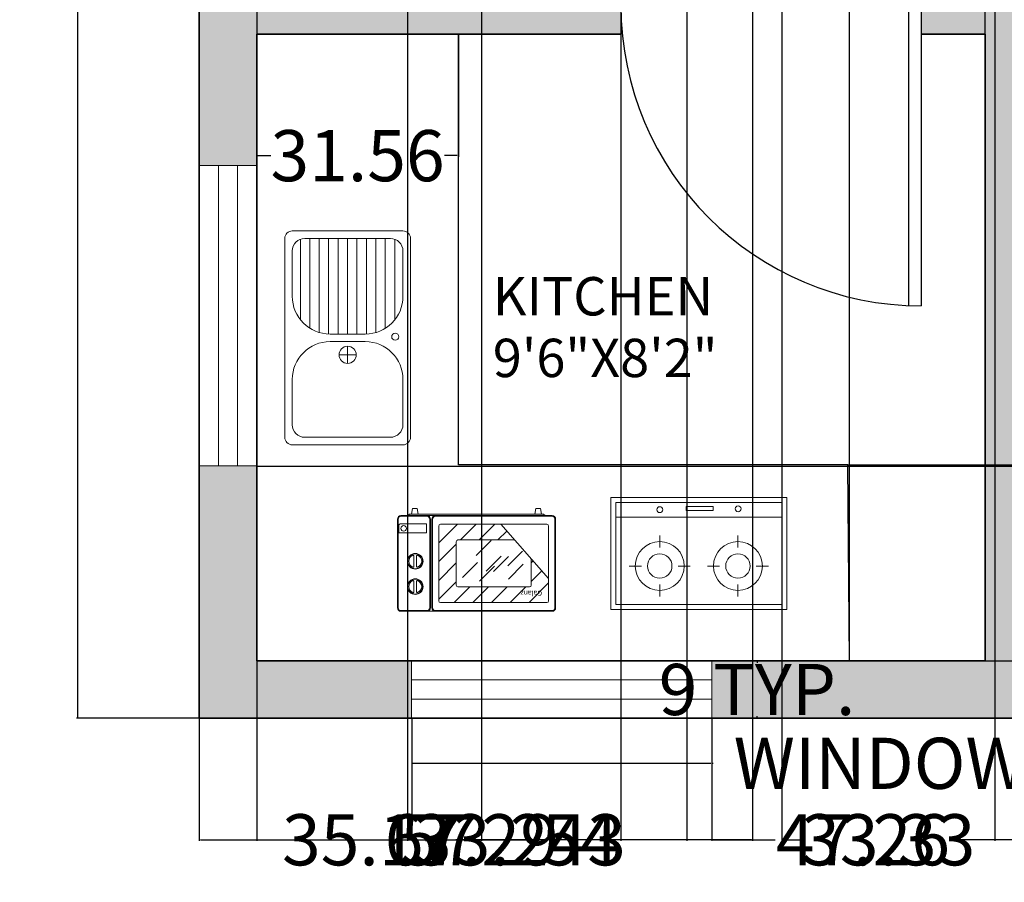
# Model space of a CAD drawing. Units: inches. Extents: x -24 to 368, y -370 to 58.
# Tile 1 of 9: x -24 to 130, y -370 to -235. Entities that reach past the tile are written whole.
import ezdxf

# ---------------------------------------------------------------- set-up
doc = ezdxf.new("R2010")
doc.units = ezdxf.units.IN
doc.header["$MEASUREMENT"] = 0
for name, color, linetype, lineweight in [('A-ANNO-DIMS', 2, 'Continuous', 18), ('A-AREA-IDEN', 7, 'Continuous', 18), ('A-EQPM', 7, 'Continuous', 15), ('A-EQPM-PATT', 7, 'Continuous', 15), ('A-FLOR-FIXT', 8, 'Continuous', 18), ('A-WALL', 7, 'Continuous', 35)]:
    doc.layers.add(name, color=color, linetype=linetype, lineweight=lineweight)
for name, color, linetype, lineweight, true_color in [('A-DOOR', 40, 'Continuous', 25, 0xf8d731), ('A-FLOR-CASE', 244, 'Continuous', 25, 0x991b1e), ('A-GLAZ', 30, 'Continuous', 18, 0xf26722), ('A-WALL-PATT', 18, 'Continuous', 13, 0x000000)]:
    doc.layers.add(name, color=color, linetype=linetype, lineweight=lineweight, true_color=true_color)
doc.styles.get("Standard").update_dxf_attribs({"font": 'arial.ttf'})
doc.dimstyles.get("Standard").update_dxf_attribs({"dimtxt": 8, "dimasz": 0.18, "dimexe": 0.18, "dimexo": 0.0625, "dimgap": 0.09, "dimtad": 0, "dimtih": 1, "dimtoh": 1, "dimdec": 4, "dimzin": 0, "dimdsep": 46, "dimlunit": 3, "dimtxsty": 'Standard', "dimcen": 0.09, "dimclre": 5, "dimclrt": 6, "dimadec": 0, "dimazin": 0, "dimtfac": 1, "dimtdec": 4, "dimtofl": 0, "dimtmove": 0, "dimatfit": 3, "dimfxl": 1, "dimtolj": 1, "dimtzin": 0, "dimarcsym": 0})

# ---------------------------------------------------------------- blocks, each defined once
blk = doc.blocks.new('WINDOW-47-JAMB-DETAIL')
for p, q in [((0, 9), (47, 9)), ((0, 0), (0, 9)), ((0, 9), (0, 4.5)), ((47, 9), (47, 0)), ((0, 6), (47, 6)), ((0, 3), (47, 3)), ((47, 0), (0, 0))]:
    blk.add_line(p, q)
blk = doc.blocks.new('WINDOW-47')
for p, q in [((0, 47), (0, 0)), ((0, 47), (9, 47)), ((3, 47), (3, 0)), ((6, 47), (6, 0)), ((9, 0), (9, 47)), ((0, 0), (9, 0))]:
    blk.add_line(p, q)
blk = doc.blocks.new('DOOR-SINGLE-47')
for p, q in [((0, 0), (0, 47)), ((2, 0), (2, 47)), ((47, 0), (0, 0))]:
    blk.add_line(p, q)
blk.add_arc((0, 0), 47, 0, 90)
blk = doc.blocks.new('*D15')
at = {"layer": 'A-ANNO-DIMS', "color": 5, "lineweight": -2, "transparency": 16777216}
for p, q in [((37.41, -344.42), (37.41, -351.59)), ((84.41, -344.42), (84.41, -351.59))]:
    blk.add_line(p, q, dxfattribs=at)
at = {"layer": 'A-ANNO-DIMS', "color": 0, "lineweight": -2, "transparency": 16777216}
for p, q in [((37.59, -351.41), (84.23, -351.41)), ((84.41, -351.41), (84.59, -351.41))]:
    blk.add_line(p, q, dxfattribs=at)
at = {"layer": 'A-ANNO-DIMS', "color": 0, "transparency": 16777216}
for points in [[(37.59, -351.38), (37.59, -351.44), (37.41, -351.41)], [(84.23, -351.38), (84.23, -351.44), (84.41, -351.41)]]:
    blk.add_solid(points, dxfattribs=at)
at = {"layer": 'Defpoints', "color": 0, "transparency": 16777216}
for p in [(37.41, -344.36), (84.41, -344.36), (84.41, -351.41)]:
    blk.add_point(p, dxfattribs=at)
at = {"layer": 'A-ANNO-DIMS', "color": 6, "transparency": 16777216, "insert": (130.38, -351.41), "char_height": 8, "attachment_point": 5}
blk.add_mtext('\\A1;WINDOW 47 TYP.', dxfattribs=at)
blk = doc.blocks.new('*D16')
at = {"layer": 'A-ANNO-DIMS', "color": 5, "lineweight": -2, "transparency": 16777216}
for p, q in [((84.47, -335.36), (91.64, -335.36)), ((84.47, -344.36), (91.64, -344.36))]:
    blk.add_line(p, q, dxfattribs=at)
at = {"layer": 'A-ANNO-DIMS', "color": 0, "lineweight": -2, "transparency": 16777216}
for p, q in [((91.46, -335.54), (91.46, -335.68)), ((91.46, -344.18), (91.46, -344.03))]:
    blk.add_line(p, q, dxfattribs=at)
at = {"layer": 'A-ANNO-DIMS', "color": 0, "transparency": 16777216}
for points in [[(91.43, -335.54), (91.49, -335.54), (91.46, -335.36)], [(91.43, -344.18), (91.49, -344.18), (91.46, -344.36)]]:
    blk.add_solid(points, dxfattribs=at)
at = {"layer": 'Defpoints', "color": 0, "transparency": 16777216}
for p in [(84.41, -335.36), (91.46, -335.36), (84.41, -344.36)]:
    blk.add_point(p, dxfattribs=at)
at = {"layer": 'A-ANNO-DIMS', "color": 6, "transparency": 16777216, "insert": (91.46, -339.86), "char_height": 8, "attachment_point": 5}
blk.add_mtext('\\A1;9 TYP.', dxfattribs=at)
blk = doc.blocks.new('*D26')
at = {"layer": 'A-ANNO-DIMS', "color": 5, "lineweight": -2, "transparency": 16777216}
for p, q in [((4.1, 33.64), (-15.03, 33.64)), ((4.1, -344.36), (-15.03, -344.36))]:
    blk.add_line(p, q, dxfattribs=at)
at = {"layer": 'A-ANNO-DIMS', "color": 0, "lineweight": -2, "transparency": 16777216}
for p, q in [((-14.85, 33.46), (-14.85, -151.18)), ((-14.85, -344.18), (-14.85, -159.53))]:
    blk.add_line(p, q, dxfattribs=at)
at = {"layer": 'A-ANNO-DIMS', "color": 0, "transparency": 16777216}
for points in [[(-14.88, 33.46), (-14.82, 33.46), (-14.85, 33.64)], [(-14.88, -344.18), (-14.82, -344.18), (-14.85, -344.36)]]:
    blk.add_solid(points, dxfattribs=at)
at = {"layer": 'Defpoints', "color": 0, "transparency": 16777216}
for p in [(-14.85, 33.64), (4.16, 33.64), (4.16, -344.36)]:
    blk.add_point(p, dxfattribs=at)
at = {"layer": 'A-ANNO-DIMS', "color": 6, "transparency": 16777216, "insert": (-14.85, -155.36), "char_height": 8, "attachment_point": 5}
blk.add_mtext('\\A1;378', dxfattribs=at)
blk = doc.blocks.new('*D27')
at = {"layer": 'A-ANNO-DIMS', "color": 5, "lineweight": -2, "transparency": 16777216}
for p, q in [((4.16, -344.42), (4.16, -363.55)), ((37.41, -344.42), (37.41, -363.55))]:
    blk.add_line(p, q, dxfattribs=at)
at = {"layer": 'A-ANNO-DIMS', "color": 0, "lineweight": -2, "transparency": 16777216}
for p, q in [((4.34, -363.37), (37.23, -363.37)), ((37.41, -363.37), (37.59, -363.37))]:
    blk.add_line(p, q, dxfattribs=at)
at = {"layer": 'A-ANNO-DIMS', "color": 0, "transparency": 16777216}
for points in [[(4.34, -363.34), (4.34, -363.4), (4.16, -363.37)], [(37.23, -363.34), (37.23, -363.4), (37.41, -363.37)]]:
    blk.add_solid(points, dxfattribs=at)
at = {"layer": 'Defpoints', "color": 0, "transparency": 16777216}
for p in [(4.16, -344.36), (37.41, -344.36), (37.41, -363.37)]:
    blk.add_point(p, dxfattribs=at)
at = {"layer": 'A-ANNO-DIMS', "color": 6, "transparency": 16777216, "insert": (54.28, -363.37), "char_height": 8, "attachment_point": 5}
blk.add_mtext('\\A1;33.243', dxfattribs=at)
blk = doc.blocks.new('*D28')
at = {"layer": 'A-ANNO-DIMS', "color": 5, "lineweight": -2, "transparency": 16777216}
for p, q in [((84.41, -344.42), (84.41, -363.55)), ((131.66, -344.42), (131.66, -363.55))]:
    blk.add_line(p, q, dxfattribs=at)
at = {"layer": 'A-ANNO-DIMS', "color": 0, "lineweight": -2, "transparency": 16777216}
for p, q in [((84.59, -363.37), (94.29, -363.37)), ((131.48, -363.37), (121.78, -363.37))]:
    blk.add_line(p, q, dxfattribs=at)
at = {"layer": 'A-ANNO-DIMS', "color": 0, "transparency": 16777216}
for points in [[(84.59, -363.34), (84.59, -363.4), (84.41, -363.37)], [(131.48, -363.34), (131.48, -363.4), (131.66, -363.37)]]:
    blk.add_solid(points, dxfattribs=at)
at = {"layer": 'Defpoints', "color": 0, "transparency": 16777216}
for p in [(84.41, -344.36), (131.66, -344.36), (131.66, -363.37)]:
    blk.add_point(p, dxfattribs=at)
at = {"layer": 'A-ANNO-DIMS', "color": 6, "transparency": 16777216, "insert": (108.03, -363.37), "char_height": 8, "attachment_point": 5}
blk.add_mtext('\\A1;47.26', dxfattribs=at)
blk = doc.blocks.new('*D40')
at = {"layer": 'A-ANNO-DIMS', "color": 5, "lineweight": -2, "transparency": 16777216}
for p, q in [((13.16, 24.58), (13.16, -363.55)), ((48.33, 24.58), (48.33, -363.55))]:
    blk.add_line(p, q, dxfattribs=at)
at = {"layer": 'A-ANNO-DIMS', "color": 0, "lineweight": -2, "transparency": 16777216}
for p, q in [((13.34, -363.37), (17.16, -363.37)), ((48.15, -363.37), (44.33, -363.37))]:
    blk.add_line(p, q, dxfattribs=at)
at = {"layer": 'A-ANNO-DIMS', "color": 0, "transparency": 16777216}
for points in [[(13.34, -363.34), (13.34, -363.4), (13.16, -363.37)], [(48.15, -363.34), (48.15, -363.4), (48.33, -363.37)]]:
    blk.add_solid(points, dxfattribs=at)
at = {"layer": 'Defpoints', "color": 0, "transparency": 16777216}
for p in [(13.16, 24.64), (48.33, 24.64), (48.33, -363.37)]:
    blk.add_point(p, dxfattribs=at)
at = {"layer": 'A-ANNO-DIMS', "color": 6, "transparency": 16777216, "insert": (30.75, -363.37), "char_height": 8, "attachment_point": 5}
blk.add_mtext('\\A1;35.17', dxfattribs=at)
blk = doc.blocks.new('*D41')
at = {"layer": 'A-ANNO-DIMS', "color": 5, "lineweight": -2, "transparency": 16777216}
for p, q in [((95.33, 24.58), (95.33, -363.55)), ((128.66, 24.58), (128.66, -363.55))]:
    blk.add_line(p, q, dxfattribs=at)
at = {"layer": 'A-ANNO-DIMS', "color": 0, "lineweight": -2, "transparency": 16777216}
for p, q in [((95.51, -363.37), (98.41, -363.37)), ((128.48, -363.37), (125.58, -363.37))]:
    blk.add_line(p, q, dxfattribs=at)
at = {"layer": 'A-ANNO-DIMS', "color": 0, "transparency": 16777216}
for points in [[(95.51, -363.34), (95.51, -363.4), (95.33, -363.37)], [(128.48, -363.34), (128.48, -363.4), (128.66, -363.37)]]:
    blk.add_solid(points, dxfattribs=at)
at = {"layer": 'Defpoints', "color": 0, "transparency": 16777216}
for p in [(95.33, 24.64), (128.66, 24.64), (128.66, -363.37)]:
    blk.add_point(p, dxfattribs=at)
at = {"layer": 'A-ANNO-DIMS', "color": 6, "transparency": 16777216, "insert": (112, -363.37), "char_height": 8, "attachment_point": 5}
blk.add_mtext('\\A1;33.33', dxfattribs=at)
blk = doc.blocks.new('*D46')
at = {"layer": 'A-ANNO-DIMS', "color": 5, "lineweight": -2, "transparency": 16777216}
for p, q in [((13.22, -304.91), (341.36, -304.91)), ((13.22, -335.36), (341.36, -335.36))]:
    blk.add_line(p, q, dxfattribs=at)
at = {"layer": 'A-ANNO-DIMS', "color": 0, "lineweight": -2, "transparency": 16777216}
for p, q in [((341.18, -305.09), (341.18, -315.95)), ((341.18, -335.18), (341.18, -324.31))]:
    blk.add_line(p, q, dxfattribs=at)
at = {"layer": 'A-ANNO-DIMS', "color": 0, "transparency": 16777216}
for points in [[(341.15, -305.09), (341.21, -305.09), (341.18, -304.91)], [(341.15, -335.18), (341.21, -335.18), (341.18, -335.36)]]:
    blk.add_solid(points, dxfattribs=at)
at = {"layer": 'Defpoints', "color": 0, "transparency": 16777216}
for p in [(13.16, -304.91), (341.18, -304.91), (13.16, -335.36)]:
    blk.add_point(p, dxfattribs=at)
at = {"layer": 'A-ANNO-DIMS', "color": 6, "transparency": 16777216, "insert": (341.18, -320.13), "char_height": 8, "attachment_point": 5}
blk.add_mtext('\\A1;30.45', dxfattribs=at)
blk = doc.blocks.new('*D47')
at = {"layer": 'A-ANNO-DIMS', "color": 5, "lineweight": -2, "transparency": 16777216}
for p, q in [((36.75, -58.62), (36.75, -363.55)), ((90.75, -58.62), (90.75, -363.55))]:
    blk.add_line(p, q, dxfattribs=at)
at = {"layer": 'A-ANNO-DIMS', "color": 0, "lineweight": -2, "transparency": 16777216}
for p, q in [((36.93, -363.37), (57.95, -363.37)), ((90.57, -363.37), (69.56, -363.37))]:
    blk.add_line(p, q, dxfattribs=at)
at = {"layer": 'A-ANNO-DIMS', "color": 0, "transparency": 16777216}
for points in [[(36.93, -363.34), (36.93, -363.4), (36.75, -363.37)], [(90.57, -363.34), (90.57, -363.4), (90.75, -363.37)]]:
    blk.add_solid(points, dxfattribs=at)
at = {"layer": 'Defpoints', "color": 0, "transparency": 16777216}
for p in [(36.75, -58.55), (90.75, -58.55), (90.75, -363.37)]:
    blk.add_point(p, dxfattribs=at)
at = {"layer": 'A-ANNO-DIMS', "color": 6, "transparency": 16777216, "insert": (63.75, -363.37), "char_height": 8, "attachment_point": 5}
blk.add_mtext('\\A1;54', dxfattribs=at)
blk = doc.blocks.new('*D53')
at = {"layer": 'A-ANNO-DIMS', "color": 5, "lineweight": -2, "transparency": 16777216}
for p, q in [((13.16, -89.42), (13.16, -363.55)), ((80.45, -89.42), (80.45, -363.55))]:
    blk.add_line(p, q, dxfattribs=at)
at = {"layer": 'A-ANNO-DIMS', "color": 0, "lineweight": -2, "transparency": 16777216}
for p, q in [((13.34, -363.37), (33.19, -363.37)), ((80.27, -363.37), (60.42, -363.37))]:
    blk.add_line(p, q, dxfattribs=at)
at = {"layer": 'A-ANNO-DIMS', "color": 0, "transparency": 16777216}
for points in [[(13.34, -363.34), (13.34, -363.4), (13.16, -363.37)], [(80.27, -363.34), (80.27, -363.4), (80.45, -363.37)]]:
    blk.add_solid(points, dxfattribs=at)
at = {"layer": 'Defpoints', "color": 0, "transparency": 16777216}
for p in [(13.16, -89.36), (80.45, -89.36), (80.45, -363.37)]:
    blk.add_point(p, dxfattribs=at)
at = {"layer": 'A-ANNO-DIMS', "color": 6, "transparency": 16777216, "insert": (46.81, -363.37), "char_height": 8, "attachment_point": 5}
blk.add_mtext('\\A1;67.29', dxfattribs=at)
blk = doc.blocks.new('*D54')
at = {"layer": 'A-ANNO-DIMS', "color": 5, "lineweight": -2, "transparency": 16777216}
for p, q in [((13.16, -232.92), (13.16, -363.55)), ((70.16, -232.92), (70.16, -363.55))]:
    blk.add_line(p, q, dxfattribs=at)
at = {"layer": 'A-ANNO-DIMS', "color": 0, "lineweight": -2, "transparency": 16777216}
for p, q in [((13.34, -363.37), (35.84, -363.37)), ((69.98, -363.37), (47.48, -363.37))]:
    blk.add_line(p, q, dxfattribs=at)
at = {"layer": 'A-ANNO-DIMS', "color": 0, "transparency": 16777216}
for points in [[(13.34, -363.34), (13.34, -363.4), (13.16, -363.37)], [(69.98, -363.34), (69.98, -363.4), (70.16, -363.37)]]:
    blk.add_solid(points, dxfattribs=at)
at = {"layer": 'Defpoints', "color": 0, "transparency": 16777216}
for p in [(13.16, -232.86), (70.16, -232.86), (70.16, -363.37)]:
    blk.add_point(p, dxfattribs=at)
at = {"layer": 'A-ANNO-DIMS', "color": 6, "transparency": 16777216, "insert": (41.66, -363.37), "char_height": 8, "attachment_point": 5}
blk.add_mtext('\\A1;57', dxfattribs=at)
blk = doc.blocks.new('*D63')
at = {"layer": 'A-ANNO-DIMS', "color": 5, "lineweight": -2, "transparency": 16777216}
for p, q in [((13.16, -237.42), (13.16, -256.55)), ((44.72, -237.42), (44.72, -256.55))]:
    blk.add_line(p, q, dxfattribs=at)
at = {"layer": 'A-ANNO-DIMS', "color": 0, "lineweight": -2, "transparency": 16777216}
for p, q in [((13.34, -256.37), (15.36, -256.37)), ((44.54, -256.37), (42.53, -256.37))]:
    blk.add_line(p, q, dxfattribs=at)
at = {"layer": 'A-ANNO-DIMS', "color": 0, "transparency": 16777216}
for points in [[(13.34, -256.34), (13.34, -256.4), (13.16, -256.37)], [(44.54, -256.34), (44.54, -256.4), (44.72, -256.37)]]:
    blk.add_solid(points, dxfattribs=at)
at = {"layer": 'Defpoints', "color": 0, "transparency": 16777216}
for p in [(13.16, -237.36), (44.72, -237.36), (13.16, -256.37)]:
    blk.add_point(p, dxfattribs=at)
at = {"layer": 'A-ANNO-DIMS', "color": 6, "transparency": 16777216, "insert": (28.94, -256.37), "char_height": 8, "attachment_point": 5}
blk.add_mtext('\\A1;31.56', dxfattribs=at)
blk = doc.blocks.new('*D64')
at = {"layer": 'A-ANNO-DIMS', "color": 5, "lineweight": -2, "transparency": 16777216}
for p, q in [((105.73, -304.73), (341.36, -304.73)), ((106.02, -335.36), (341.36, -335.36))]:
    blk.add_line(p, q, dxfattribs=at)
at = {"layer": 'A-ANNO-DIMS', "color": 0, "lineweight": -2, "transparency": 16777216}
for p, q in [((341.18, -304.91), (341.18, -315.86)), ((341.18, -335.18), (341.18, -324.22))]:
    blk.add_line(p, q, dxfattribs=at)
at = {"layer": 'A-ANNO-DIMS', "color": 0, "transparency": 16777216}
for points in [[(341.15, -304.91), (341.21, -304.91), (341.18, -304.73)], [(341.15, -335.18), (341.21, -335.18), (341.18, -335.36)]]:
    blk.add_solid(points, dxfattribs=at)
at = {"layer": 'Defpoints', "color": 0, "transparency": 16777216}
for p in [(105.67, -304.73), (341.18, -304.73), (105.95, -335.36)]:
    blk.add_point(p, dxfattribs=at)
at = {"layer": 'A-ANNO-DIMS', "color": 6, "transparency": 16777216, "insert": (341.18, -320.04), "char_height": 8, "attachment_point": 5}
blk.add_mtext('\\A1;30.63', dxfattribs=at)
blk = doc.blocks.new('*D65')
at = {"layer": 'A-ANNO-DIMS', "color": 5, "lineweight": -2, "transparency": 16777216}
for p, q in [((105.95, -335.29), (105.95, 52.85)), ((127.16, -335.29), (127.16, 52.85))]:
    blk.add_line(p, q, dxfattribs=at)
at = {"layer": 'A-ANNO-DIMS', "color": 0, "lineweight": -2, "transparency": 16777216}
for p, q in [((106.13, 52.67), (126.98, 52.67)), ((127.16, 52.67), (127.34, 52.67))]:
    blk.add_line(p, q, dxfattribs=at)
at = {"layer": 'A-ANNO-DIMS', "color": 0, "transparency": 16777216}
for points in [[(106.13, 52.7), (106.13, 52.64), (105.95, 52.67)], [(126.98, 52.7), (126.98, 52.64), (127.16, 52.67)]]:
    blk.add_solid(points, dxfattribs=at)
at = {"layer": 'Defpoints', "color": 0, "transparency": 16777216}
for p in [(127.16, 52.67), (105.95, -335.36), (127.16, -335.36)]:
    blk.add_point(p, dxfattribs=at)
at = {"layer": 'A-ANNO-DIMS', "color": 6, "transparency": 16777216, "insert": (140.23, 52.67), "char_height": 8, "attachment_point": 5}
blk.add_mtext('\\A1;21.21', dxfattribs=at)

msp = doc.modelspace()

# ---------------------------------------------------------------- hatches: boundary and pattern name
at = {"layer": 'A-EQPM-PATT'}
h = msp.add_hatch(dxfattribs=at)
h.set_pattern_fill('ANSI31', color=256, scale=16.582045, style=0)
h.set_pattern_definition([(45, (-645.9693, -345.0149), (-1.4656596, 1.4656596), [])])
h.paths.add_polyline_path([(51.3569, -314.0293), (53.5154, -316.4774), (44.6502, -316.4774), (44.6324, -316.478), (44.6147, -316.4797), (44.5972, -316.4826), (44.5798, -316.4867), (44.5628, -316.4918), (44.5461, -316.4981), (44.5299, -316.5055), (44.5142, -316.5138), (44.4991, -316.5232), (44.4846, -316.5336), (44.4709, -316.5449), (44.4579, -316.5571), (44.4457, -316.5701), (44.4344, -316.5838), (44.424, -316.5983), (44.4147, -316.6134), (44.4063, -316.6291), (44.3989, -316.6453), (44.3926, -316.662), (44.3875, -316.679), (44.3834, -316.6964), (44.3805, -316.7139), (44.3788, -316.7316), (44.3782, -316.7494), (44.3782, -323.5498), (44.3788, -323.5676), (44.3805, -323.5853), (44.3834, -323.6029), (44.3875, -323.6202), (44.3926, -323.6372), (44.3989, -323.6539), (44.4063, -323.6701), (44.4147, -323.6858), (44.424, -323.7009), (44.4344, -323.7154), (44.4457, -323.7292), (44.4579, -323.7421), (44.4709, -323.7543), (44.4846, -323.7656), (44.4991, -323.776), (44.5142, -323.7854), (44.5299, -323.7938), (44.5461, -323.8011), (44.5628, -323.8074), (44.5798, -323.8125), (44.5972, -323.8166), (44.6147, -323.8195), (44.6324, -323.8212), (44.6502, -323.8218), (55.8572, -323.8218), (55.875, -323.8212), (55.8928, -323.8195), (55.9103, -323.8166), (55.9277, -323.8125), (55.9447, -323.8074), (55.9613, -323.8011), (55.9776, -323.7938), (55.9933, -323.7854), (56.0084, -323.776), (56.0228, -323.7656), (56.0366, -323.7543), (56.0496, -323.7421), (56.0618, -323.7292), (56.0731, -323.7154), (56.0834, -323.7009), (56.0928, -323.6858), (56.1012, -323.6701), (56.1086, -323.6539), (56.1148, -323.6372), (56.12, -323.6202), (56.124, -323.6029), (56.1269, -323.5853), (56.1287, -323.5676), (56.1293, -323.5498), (56.1293, -319.4421), (58.8494, -322.5274), (58.8494, -325.9979), (58.8488, -326.0157), (58.8471, -326.0334), (58.8442, -326.051), (58.8401, -326.0683), (58.835, -326.0854), (58.8287, -326.102), (58.8214, -326.1182), (58.813, -326.1339), (58.8036, -326.1491), (58.7932, -326.1635), (58.7819, -326.1773), (58.7697, -326.1903), (58.7568, -326.2024), (58.743, -326.2137), (58.7285, -326.2241), (58.7134, -326.2335), (58.6977, -326.2419), (58.6815, -326.2492), (58.6648, -326.2555), (58.6478, -326.2607), (58.6305, -326.2647), (58.6129, -326.2676), (58.5952, -326.2694), (58.5774, -326.27), (41.9301, -326.27), (41.9123, -326.2694), (41.8946, -326.2676), (41.877, -326.2647), (41.8597, -326.2607), (41.8426, -326.2555), (41.826, -326.2492), (41.8098, -326.2419), (41.7941, -326.2335), (41.7789, -326.2241), (41.7645, -326.2137), (41.7507, -326.2024), (41.7377, -326.1903), (41.7256, -326.1773), (41.7143, -326.1635), (41.7039, -326.1491), (41.6945, -326.1339), (41.6861, -326.1182), (41.6788, -326.102), (41.6725, -326.0854), (41.6673, -326.0683), (41.6633, -326.051), (41.6604, -326.0334), (41.6586, -326.0157), (41.6581, -325.9979), (41.6581, -314.3013), (41.6586, -314.2835), (41.6604, -314.2658), (41.6633, -314.2482), (41.6673, -314.2309), (41.6725, -314.2138), (41.6788, -314.1972), (41.6861, -314.181), (41.6945, -314.1653), (41.7039, -314.1502), (41.7143, -314.1357), (41.7256, -314.1219), (41.7377, -314.1089), (41.7507, -314.0968), (41.7645, -314.0855), (41.7789, -314.0751), (41.7941, -314.0657), (41.8098, -314.0573), (41.826, -314.05), (41.8426, -314.0437), (41.8597, -314.0385), (41.877, -314.0345), (41.8946, -314.0316), (41.9123, -314.0299), (41.9301, -314.0293)])
at = {"layer": 'A-WALL-PATT'}
h = msp.add_hatch(color=256, dxfattribs=at)
h.dxf.hatch_style = 1
h.paths.add_polyline_path([(13.1621, -93.8573), (80.4499, -93.8573), (80.4499, -89.3573), (13.1621, -89.3573), (13.1621, -61.0987), (4.1621, -61.0987), (4.1621, -149.8573), (13.1621, -149.8573)])
h.paths.add_polyline_path([(146.5668, -27.3573), (133.1621, -27.3573), (133.1621, 10.3323), (133.1272, 10.3313), (133.1621, 24.6427), (139.8141, 24.6427), (139.8141, 33.6427), (95.3329, 33.6427), (95.3329, 24.6427), (128.6621, 24.6427), (128.6621, -89.3573), (127.4499, -89.3573), (127.4499, -93.8573), (133.1621, -93.8573), (133.1621, -31.8573), (146.5668, -31.8573)])
h.paths.add_polyline_path([(197.6621, 24.6427), (236.2134, 24.6427), (236.2134, 33.6427), (169.8141, 33.6427), (169.8141, 24.6427), (193.1621, 24.6427), (193.1621, -27.3573), (181.5668, -27.3573), (181.5668, -31.8573), (193.1621, -31.8573), (193.1621, -95.8573), (199.2127, -95.8573), (199.2127, -91.3573), (197.6621, -91.3573)])
h.paths.add_polyline_path([(322.1621, -52.531), (313.1621, -52.531), (313.1621, -91.3573), (246.2127, -91.3573), (246.2127, -95.8573), (246.6621, -95.8573), (246.6621, -104.9077), (251.1621, -104.9077), (251.1621, -95.8573), (313.1621, -95.8573), (313.1621, -105.6922), (317.6621, -105.6922), (322.1621, -105.6922)])
h.paths.add_polyline_path([(322.1621, -135.6922), (313.1621, -135.6922), (313.1621, -147.8573), (251.1621, -147.8573), (251.1621, -139.9077), (246.6621, -139.9077), (246.6621, -147.8573), (199.43, -147.8573), (199.43, -152.3573), (313.1621, -152.3573), (313.1621, -194.6142), (317.6621, -194.6142), (322.1621, -194.6142)])
h.paths.add_polyline_path([(322.1621, -241.6142), (313.1621, -241.6142), (313.1621, -275.3573), (287.3912, -275.3573), (287.3912, -279.8573), (313.1621, -279.8573), (313.1621, -335.3573), (298.077, -335.3573), (298.077, -344.3573), (322.1621, -344.3573)])
h.paths.add_polyline_path([(263.077, -335.3573), (241.1621, -335.3573), (241.1621, -279.8573), (252.3912, -279.8573), (252.3912, -275.3573), (236.6621, -275.3573), (236.6621, -298.8573), (234.5689, -298.8573), (234.5689, -303.3573), (236.6621, -303.3573), (236.6621, -344.3573), (263.077, -344.3573), (263.077, -339.8573)])
h.paths.add_polyline_path([(175.5689, -298.8573), (131.6621, -298.8573), (131.6621, -152.3573), (164.43, -152.3573), (164.43, -147.8573), (127.1621, -147.8573), (127.1621, -232.8573), (117.1621, -232.8573), (117.1621, -237.3573), (127.1621, -237.3573), (127.1621, -335.3573), (84.4055, -335.3573), (84.4055, -344.3573), (131.6621, -344.3573), (131.6621, -303.3573), (175.5689, -303.3573)])
h.paths.add_polyline_path([(70.1621, -232.8573), (13.1621, -232.8573), (13.1621, -196.8573), (4.1621, -196.8573), (4.1621, -257.9061), (13.1621, -257.9061), (13.1621, -237.3573), (70.1621, -237.3573)])
h.paths.add_polyline_path([(13.1621, -304.9061), (4.1621, -304.9061), (4.1621, -344.3573), (37.4055, -344.3573), (37.4055, -335.3573), (13.1621, -335.3573)])
h.paths.add_polyline_path([(322.1621, 33.6427), (283.2134, 33.6427), (283.2134, 24.6427), (313.1621, 24.6427), (313.1621, 11.9273), (313.4656, 11.629), (313.1621, 11.629), (313.1621, -5.531), (322.1621, -5.531)])
h.paths.add_polyline_path([(48.3329, 33.6427), (4.1621, 33.6427), (4.1621, -14.0987), (13.1621, -14.0987), (13.1621, 24.6427), (48.3329, 24.6427)])

# ---------------------------------------------------------------- linework, layer by layer
at = {"layer": 'A-DOOR'}
for p, q in [((70.1621, -232.8573), (70.1621, -237.3573)), ((117.1621, -232.8573), (117.1621, -237.3573)), ((70.1621, -237.3573), (70.1621, -237.3573))]:
    msp.add_line(p, q, dxfattribs=at)
at = {"layer": 'A-EQPM'}
for p, q in [((96.133, -309.829), (68.577, -309.829)), ((68.577, -327.3287), (68.577, -309.829)), ((95.3673, -310.5946), (69.3427, -310.5946)), ((69.3427, -326.563), (69.3427, -310.5946)), ((80.3605, -311.8729), (80.3605, -311.2656)), ((80.3605, -311.2656), (84.5816, -311.2656)), ((84.5816, -311.2656), (84.5816, -311.8729)), ((95.3673, -326.563), (95.3673, -310.5946)), ((96.133, -327.3287), (96.133, -309.829)), ((39.8084, -312.6692), (35.7281, -312.6692)), ((39.8084, -312.778), (35.7281, -312.778)), ((36.8162, -312.6692), (37.0882, -312.4516)), ((38.7203, -312.4516), (37.0882, -312.4516)), ((37.3929, -312.4516), (37.5234, -311.5811)), ((38.2851, -311.5811), (37.5234, -311.5811)), ((38.4156, -312.4516), (38.2851, -311.5811)), ((56.4013, -312.4516), (38.7203, -312.4516)), ((41.114, -312.6692), (39.8084, -312.6692)), ((59.3934, -312.6692), (41.114, -312.6692)), ((59.3934, -312.778), (41.114, -312.778)), ((58.0334, -312.4516), (56.4013, -312.4516)), ((56.7059, -312.4516), (56.8365, -311.5811)), ((57.5981, -311.5811), (56.8365, -311.5811)), ((57.7287, -312.4516), (57.5981, -311.5811)), ((58.0334, -312.4516), (58.3054, -312.6692)), ((84.5816, -311.8729), (80.3605, -311.8729)), ((35.1841, -313.2132), (35.1841, -327.086)), ((35.2929, -313.2132), (35.2929, -327.086)), ((35.4031, -314.1945), (35.4031, -315.337)), ((39.7554, -313.9769), (35.6207, -313.9769)), ((39.7554, -315.337), (39.7554, -313.9769)), ((40.2436, -313.2132), (40.2436, -327.086)), ((40.3524, -313.2132), (40.3524, -327.086)), ((40.57, -313.2132), (40.57, -327.086)), ((40.6788, -313.2132), (40.6788, -327.086)), ((41.6581, -314.3013), (41.6581, -325.9979)), ((58.5774, -314.0293), (41.9301, -314.0293)), ((58.8494, -322.5274), (51.3569, -314.0293)), ((58.8494, -325.9979), (58.8494, -314.3013)), ((59.8287, -327.086), (59.8287, -313.2132)), ((59.9375, -327.086), (59.9375, -313.2132)), ((95.3673, -312.8917), (69.3427, -312.8917)), ((35.4031, -315.337), (39.7554, -315.337)), ((76.2337, -317.6784), (76.2337, -315.7642)), ((88.4763, -317.6784), (88.4763, -315.7642)), ((44.3782, -316.7494), (44.3782, -323.5498)), ((53.5154, -316.4774), (44.6502, -316.4774)), ((49.8454, -316.5443), (47.5091, -318.8807)), ((37.7517, -320.6454), (37.7517, -318.973)), ((38.1869, -320.6454), (38.1869, -318.973)), ((54.7781, -318.2112), (52.4417, -320.5476)), ((47.6971, -319.9957), (45.3608, -322.3321)), ((51.404, -319.0277), (49.0676, -321.364)), ((52.5668, -319.0744), (50.2305, -321.4107)), ((54.8791, -320.2693), (52.5428, -322.6057)), ((56.1293, -323.5498), (56.1293, -319.4421)), ((50.3509, -320.585), (48.0145, -322.9214)), ((73.3624, -320.5497), (71.4483, -320.5497)), ((81.0192, -320.5497), (79.105, -320.5497)), ((85.605, -320.5497), (83.6908, -320.5497)), ((93.2617, -320.5497), (91.3475, -320.5497)), ((37.7517, -324.6113), (37.7517, -322.9389)), ((38.1869, -324.6113), (38.1869, -322.9389)), ((76.2337, -325.3351), (76.2337, -323.4209)), ((88.4763, -325.3351), (88.4763, -323.4209)), ((44.6502, -323.8218), (55.8572, -323.8218)), ((41.9301, -326.27), (58.5774, -326.27)), ((95.3673, -326.563), (69.3427, -326.563)), ((39.8084, -327.5212), (35.7281, -327.5212)), ((39.8084, -327.63), (35.7281, -327.63)), ((41.114, -327.63), (39.0808, -327.63)), ((41.114, -327.5212), (59.3934, -327.5212)), ((41.114, -327.63), (59.3934, -327.63)), ((96.133, -327.3287), (68.577, -327.3287))]:
    msp.add_line(p, q, dxfattribs=at)
for centre, radius in [((76.2418, -311.738), 0.4594), ((88.4977, -311.603), 0.4594), ((36.1595, -314.6686), 0.4339), ((76.2337, -320.5497), 3.8284), ((88.4763, -320.5497), 3.8284), ((37.9693, -319.8092), 1.2241), ((37.9693, -319.8092), 1.1697), ((76.2337, -320.5497), 1.9142), ((88.4763, -320.5497), 1.9142), ((37.9693, -323.7751), 1.2241), ((37.9693, -323.7751), 1.1697)]:
    msp.add_circle(centre, radius, dxfattribs=at)
for centre, radius, start, end in [((35.7281, -313.2132), 0.544, 90, 180), ((35.7281, -313.2132), 0.4352, 90, 180), ((39.8084, -313.2132), 0.544, 0, 90), ((39.8084, -313.2132), 0.4352, 0, 90), ((41.114, -313.2132), 0.544, 90, 180), ((41.114, -313.2132), 0.4352, 90, 180), ((59.3934, -313.2132), 0.544, 0, 90), ((59.3934, -313.2132), 0.4352, 0, 90), ((35.6207, -314.1945), 0.2176, 90, 180), ((41.9301, -314.3013), 0.272, 90, 180), ((58.5774, -314.3013), 0.272, 0, 90), ((44.6502, -316.7494), 0.272, 90, 180), ((37.9693, -319.8092), 1.0065, 111.323686, 248.676314), ((37.6429, -318.973), 0.1088, 0, 111.323686), ((38.2957, -318.973), 0.1088, 68.676314, 180), ((37.9693, -319.8092), 1.0065, 291.323686, 68.676314), ((37.6429, -320.6454), 0.1088, 248.676314, 0), ((38.2957, -320.6454), 0.1088, 180, 291.323686), ((37.9693, -323.7751), 1.0065, 111.323686, 248.676314), ((37.6429, -322.9389), 0.1088, 0, 111.323686), ((38.2957, -322.9389), 0.1088, 68.676314, 180), ((37.9693, -323.7751), 1.0065, 291.323686, 68.676314), ((44.6502, -323.5498), 0.272, 180, 270), ((55.8572, -323.5498), 0.272, 270, 0), ((37.6429, -324.6113), 0.1088, 248.676314, 0), ((38.2957, -324.6113), 0.1088, 180, 291.323686), ((41.9301, -325.9979), 0.272, 180, 270), ((58.5774, -325.9979), 0.272, 270, 0), ((35.7281, -327.086), 0.544, 180, 270), ((35.7281, -327.086), 0.4352, 180, 270), ((39.8084, -327.086), 0.544, 270, 0), ((39.8084, -327.086), 0.4352, 270, 0), ((41.114, -327.086), 0.544, 180, 270), ((41.114, -327.086), 0.4352, 180, 270), ((59.3934, -327.086), 0.544, 270, 0), ((59.3934, -327.086), 0.4352, 270, 0)]:
    msp.add_arc(centre, radius, start, end, dxfattribs=at)
at = {"layer": 'A-FLOR-CASE'}
for p, q in [((44.7246, -304.7252), (44.7246, -237.3573)), ((105.6669, -304.7252), (44.7246, -304.7252)), ((105.953, -335.3573), (105.6669, -304.7252))]:
    msp.add_line(p, q, dxfattribs=at)
at = {"layer": 'A-FLOR-FIXT'}
for p, q in [((36.0477, -268.1322), (18.7249, -268.1322)), ((17.5438, -269.3133), (17.5438, -300.4156)), ((19.9866, -269.4526), (19.9866, -281.9943)), ((34.0792, -269.3133), (20.6934, -269.3133)), ((21.4629, -269.3133), (21.4629, -283.3412)), ((22.9393, -269.3133), (22.9393, -284.0208)), ((24.4157, -269.3133), (24.4157, -284.2686)), ((25.8921, -269.3133), (25.8921, -284.2739)), ((27.3684, -269.3133), (27.3684, -284.2739)), ((28.8448, -269.3133), (28.8448, -284.2739)), ((30.3212, -269.3133), (30.3212, -284.2724)), ((31.7976, -269.3133), (31.7976, -284.0427)), ((33.2739, -269.3133), (33.2739, -283.3862)), ((34.7503, -269.4241), (34.7503, -282.0833)), ((37.2288, -269.3133), (37.2288, -300.4156)), ((18.7249, -278.3684), (18.7249, -271.2818)), ((36.0477, -278.3684), (36.0477, -271.2818)), ((30.1422, -284.2739), (24.6304, -284.2739)), ((30.1422, -285.455), (24.6304, -285.455)), ((27.3863, -288.8668), (27.3863, -286.1842)), ((28.7276, -287.5255), (26.045, -287.5255)), ((18.7249, -291.3605), (18.7249, -298.4471)), ((36.0477, -291.3605), (36.0477, -298.4471)), ((34.0792, -300.4156), (20.6934, -300.4156)), ((36.0477, -301.5967), (18.7249, -301.5967))]:
    msp.add_line(p, q, dxfattribs=at)
for centre, radius in [((34.8362, -284.6892), 0.5539), ((27.3863, -287.5255), 1.3413)]:
    msp.add_circle(centre, radius, dxfattribs=at)
for centre, radius, start, end in [((18.7249, -269.3133), 1.1811, 90, 180), ((36.0477, -269.3133), 1.1811, 0, 90), ((20.6934, -271.2818), 1.9685, 90, 180), ((34.0792, -271.2818), 1.9685, 0, 90), ((24.6304, -278.3684), 5.9055, 180, 270), ((30.1422, -278.3684), 5.9055, 270, 0), ((24.6304, -291.3605), 5.9055, 90, 180), ((30.1422, -291.3605), 5.9055, 0, 90), ((20.6934, -298.4471), 1.9685, 180, 270), ((34.0792, -298.4471), 1.9685, 270, 0), ((18.7249, -300.4156), 1.1811, 180, 270), ((36.0477, -300.4156), 1.1811, 270, 0)]:
    msp.add_arc(centre, radius, start, end, dxfattribs=at)
at = {"layer": 'A-WALL'}
for p, q in [((4.1621, -344.3573), (4.1621, 33.6427)), ((13.1621, -335.3573), (13.1621, -237.3573)), ((70.1621, -237.3573), (13.1621, -237.3573)), ((127.1621, -237.3573), (117.1621, -237.3573)), ((127.1621, -335.3573), (127.1621, -237.3573)), ((127.1621, -335.3573), (13.1621, -335.3573)), ((322.1621, -344.3573), (4.1621, -344.3573))]:
    msp.add_line(p, q, dxfattribs=at)

# ---------------------------------------------------------------- block references
at = {"layer": 'A-DOOR', "rotation": 180}
msp.add_blockref('DOOR-SINGLE-47', (117.1618, -232.8576), dxfattribs=at)
at = {"layer": 'A-GLAZ'}
for name, p in [('WINDOW-47', (4.162, -304.906)), ('WINDOW-47-JAMB-DETAIL', (37.4051, -344.357))]:
    msp.add_blockref(name, p, dxfattribs=at)

# ---------------------------------------------------------------- texts
at = {"layer": 'A-AREA-IDEN'}
for s, p in [('KITCHEN', (50.1063, -281.3643)), ('9\'6"X8\'2"', (50.1063, -291.0028))]:
    msp.add_text(s, height=6, dxfattribs=at).set_placement(p)
at = {"layer": 'A-EQPM'}
msp.add_text('Galanz', height=0.77992, rotation=180, dxfattribs=at).set_placement((57.8248, -324.423))

# ---------------------------------------------------------------- dimensions: what is measured, and where the dimension line sits
at = {"layer": 'A-ANNO-DIMS'}
for base, p1, p2, override, picture, middle in [((127.1621, 52.6658), (105.953, -335.3573), (127.1621, -335.3573), {"dimdec": 2, "dimlfac": 1, "dimrnd": 0, "dimzin": 0, "dimdsep": 46, "dimlunit": 2}, '*D65', (140.2261, 52.6658)), ((48.3329, -363.3723), (13.1621, 24.6427), (48.3329, 24.6427), {"dimdec": 2, "dimlfac": 1, "dimrnd": 0, "dimzin": 0, "dimdsep": 46, "dimlunit": 2}, '*D40', (30.7475, -363.3723)), ((128.6621, -363.3723), (95.3329, 24.6427), (128.6621, 24.6427), {"dimdec": 2, "dimlfac": 1, "dimrnd": 0, "dimzin": 0, "dimdsep": 46, "dimlunit": 2}, '*D41', (111.9975, -363.3723)), ((90.7545, -363.3723), (36.7545, -58.5547), (90.7545, -58.5547), {"dimdec": 0, "dimlfac": 1, "dimrnd": 0, "dimzin": 0, "dimdsep": 46, "dimlunit": 2}, '*D47', (63.7545, -363.3723)), ((80.4499, -363.3723), (13.1621, -89.3573), (80.4499, -89.3573), {"dimdec": 2, "dimlfac": 1, "dimrnd": 0, "dimzin": 0, "dimdsep": 46, "dimlunit": 2}, '*D53', (46.806, -363.3723)), ((70.1621, -363.3723), (13.1621, -232.8573), (70.1621, -232.8573), {"dimdec": 0, "dimlfac": 1, "dimrnd": 0, "dimzin": 0, "dimdsep": 46, "dimlunit": 2}, '*D54', (41.6621, -363.3723)), ((37.4055, -363.3723), (4.1621, -344.3573), (37.4055, -344.3573), {"dimdec": 3, "dimlfac": 1, "dimrnd": 0, "dimzin": 0, "dimdsep": 46, "dimlunit": 2}, '*D27', (54.2785, -363.3723)), ((131.6621, -363.3723), (84.4055, -344.3573), (131.6621, -344.3573), {"dimdec": 2, "dimlfac": 1, "dimrnd": 0, "dimzin": 0, "dimdsep": 46, "dimlunit": 2}, '*D28', (108.0338, -363.3723))]:
    dim = msp.add_linear_dim(base=base, p1=p1, p2=p2, dimstyle='Standard', override=override, dxfattribs=at)
    dim.commit()
    dim.dimension.update_dxf_attribs({"geometry": picture, "text_midpoint": middle})
for base, p1, p2, angle, override, picture, middle in [((-14.8529, 33.6427), (4.1621, -344.3573), (4.1621, 33.6427), 90, {"dimdec": 0, "dimlfac": 1, "dimrnd": 0, "dimzin": 0, "dimdsep": 46, "dimlunit": 2}, '*D26', (-14.8529, -155.3573)), ((13.1621, -256.3723), (44.7246, -237.3573), (13.1621, -237.3573), 180, {"dimdec": 2, "dimlfac": 1, "dimrnd": 0, "dimzin": 0, "dimdsep": 46, "dimlunit": 2}, '*D63', (28.9434, -256.3723)), ((341.1771, -304.9061), (13.1621, -335.3573), (13.1621, -304.9061), 90, {"dimdec": 2, "dimlfac": 1, "dimrnd": 0, "dimzin": 0, "dimdsep": 46, "dimlunit": 2}, '*D46', (341.1771, -320.1317)), ((341.1771, -304.7252), (105.953, -335.3573), (105.6669, -304.7252), 90, {"dimdec": 2, "dimlfac": 1, "dimrnd": 0, "dimzin": 0, "dimdsep": 46, "dimlunit": 2}, '*D64', (341.1771, -320.0412))]:
    dim = msp.add_linear_dim(base=base, p1=p1, p2=p2, angle=angle, dimstyle='Standard', override=override, dxfattribs=at)
    dim.commit()
    dim.dimension.update_dxf_attribs({"geometry": picture, "text_midpoint": middle})
dim = msp.add_linear_dim(base=(91.4555, -335.3573), p1=(84.4055, -344.3573), p2=(84.4055, -335.3573), angle=90, text='<> TYP.', dimstyle='Standard', override={"dimdec": 0, "dimlfac": 1, "dimrnd": 0, "dimzin": 0, "dimdsep": 46, "dimlunit": 2}, dxfattribs=at)
dim.commit()
dim.dimension.update_dxf_attribs({"geometry": '*D16', "text_midpoint": (91.4555, -339.8573)})
dim = msp.add_linear_dim(base=(84.4055, -351.4073), p1=(37.4055, -344.3573), p2=(84.4055, -344.3573), text='WINDOW <> TYP.', dimstyle='Standard', override={"dimdec": 0, "dimlfac": 1, "dimrnd": 0, "dimzin": 0, "dimdsep": 46, "dimlunit": 2}, dxfattribs=at)
dim.commit()
dim.dimension.update_dxf_attribs({"geometry": '*D15', "text_midpoint": (130.3808, -351.4073)})

doc.saveas('drawing.dxf')
